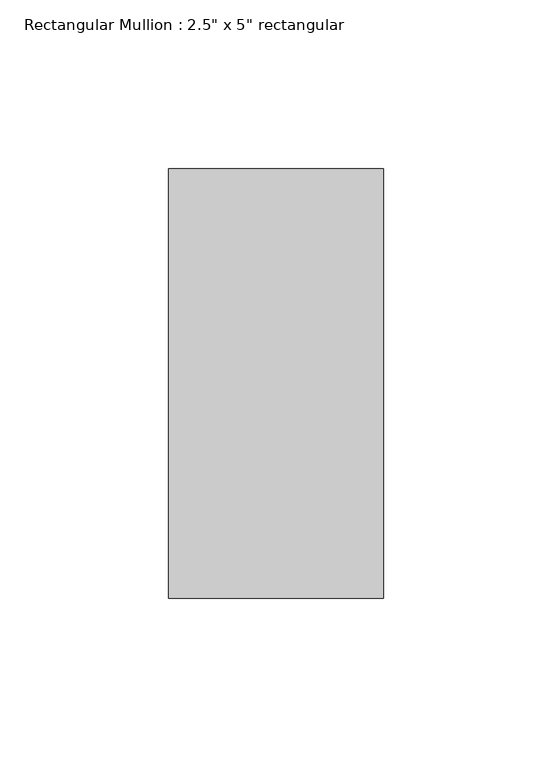
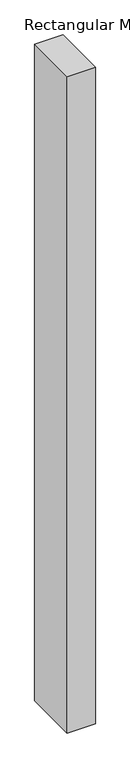
"""IFC4 building model written with IfcOpenShell, lengths in millimetres: member geometry."""

from ifc_helpers import new_model, si_unit, frame, origin, place, context, project, spatial, polyline, outline, extrude, source, transform, mapped, element, save


def member_3b277a63(model_context):
    return source(origin(), model_context, "Body", "SweptSolid", [
        extrude(outline(polyline([(0.0, 63.5), (0.0, -63.5), (-63.5, -63.5), (-63.5, 63.5), (0.0, 63.5)])), frame((0.0, 0.0, -1566.7320436), z_axis=(0.0, 0.0, 1.0), x_axis=(1.0, 0.0, 0.0)), (0.0, 0.0, 1.0), 1566.7320436),
    ])


if __name__ == "__main__":
    model = new_model("IFC4")
    model_context = context("Model", 3, world=origin())
    ifc_project = project(units=[si_unit("LENGTHUNIT", "METRE", prefix="MILLI")], contexts=[model_context])
    site = spatial("IfcSite", under=ifc_project)
    building = spatial("IfcBuilding", under=site)
    placement = place(None, origin())
    member_shape = member_3b277a63(model_context)
    element("IfcMember", 1, ObjectType="Rectangular Mullion : 2.5\" x 5\" rectangular", at=placement, inside=building, context=model_context, shape_type="MappedRepresentation", body=[
        mapped(member_shape, transform((0.0, 0.0, 0.0), x_axis=(1.0, 0.0, 0.0), y_axis=(0.0, 1.0, 0.0), z_axis=(0.0, 0.0, 1.0))),
    ])
    save(model, "model.ifc")

# Revit data of these elements
# Type "Rectangular Mullion : 2.5\" x 5\" rectangular"
#   built-in parameter 1007304 = 0.416667 (stored number, unit not read)
#   built-in parameter 1007301 = 0.104167 (stored number, unit not read)
#   built-in parameter 1007300 = 0.104167 (stored number, unit not read)
# Element 1 (IfcMember, "Rectangular Mullion : 2.5\" x 5\" rectangular")
#   Materials on its faces: "Aluminum"
# Materials
#   "Aluminum": class "Metal", colour RGB 247 247 247, transparency 0, Description = "Aluminum 6061", Cost = 0
